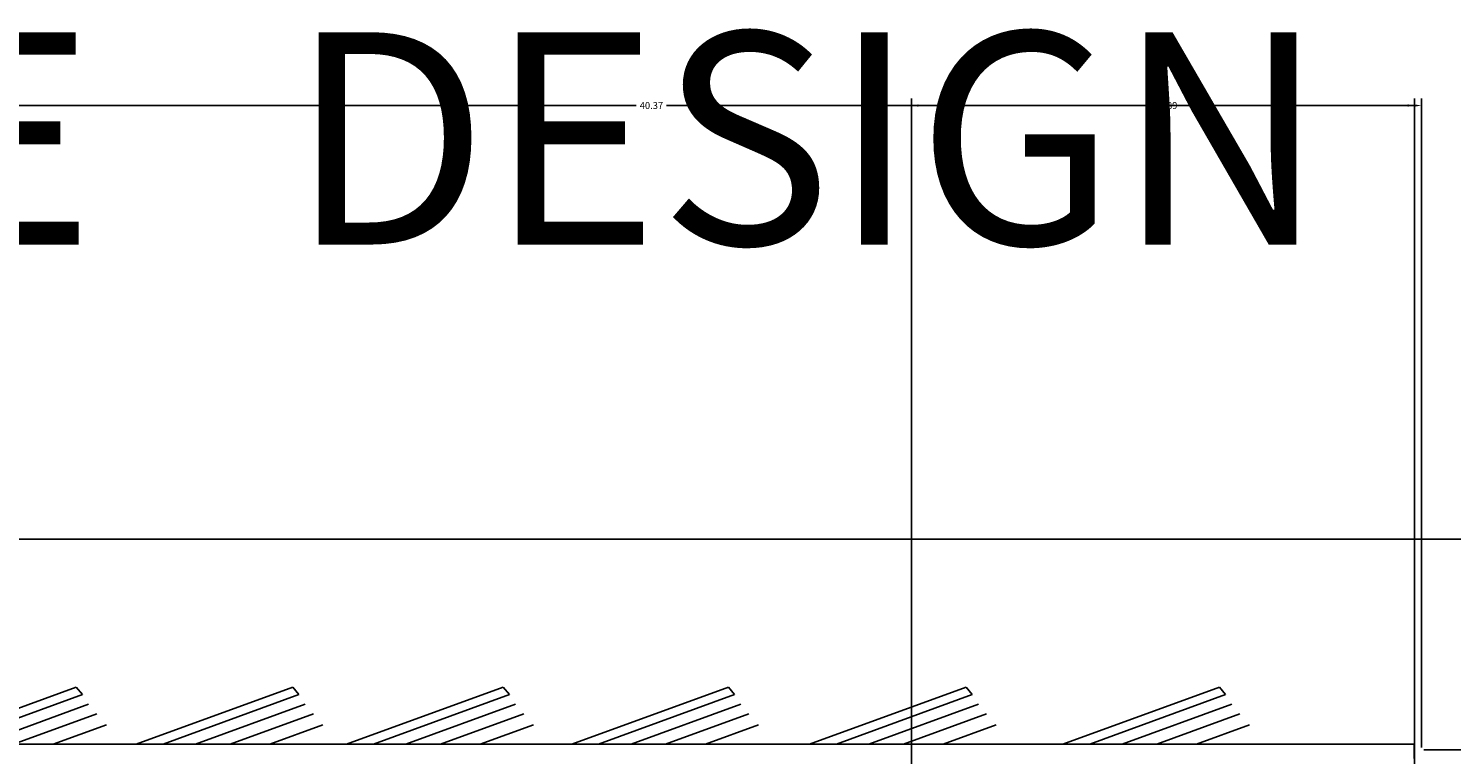
# Model space of a CAD drawing. Units: inches. Extents: x -117 to 121, y -77 to 40.
# Tile 36 of 45: x 34 to 72, y 21 to 40. Entities that reach past the tile are written whole.
import ezdxf

# ---------------------------------------------------------------- set-up
doc = ezdxf.new("R2010")
doc.units = ezdxf.units.IN
doc.header["$MEASUREMENT"] = 0
for name, color, linetype, lineweight in [('A-ANNO-DIMS', 2, 'Continuous', 18), ('A-ANNO-TEXT', 7, 'Continuous', 25), ('A-ELEV', 7, 'Continuous', 25)]:
    doc.layers.add(name, color=color, linetype=linetype, lineweight=lineweight)
doc.styles.get("Standard").update_dxf_attribs({"font": 'arial.ttf'})
doc.dimstyles.get("Standard").update_dxf_attribs({"dimtxt": 0.18, "dimasz": 0.18, "dimexe": 0.18, "dimexo": 0.0625, "dimgap": 0.09, "dimtad": 0, "dimtih": 1, "dimtoh": 1, "dimdec": 4, "dimzin": 0, "dimdsep": 46, "dimtxsty": 'Standard', "dimcen": 0.09, "dimadec": 0, "dimazin": 0, "dimtfac": 1, "dimtdec": 4, "dimtofl": 0, "dimtmove": 0, "dimatfit": 3, "dimfxl": 1, "dimtolj": 1, "dimtzin": 0, "dimarcsym": 0})

# ---------------------------------------------------------------- blocks, each defined once
blk = doc.blocks.new('*D11')
at = {"layer": 'A-ANNO-DIMS', "color": 0, "lineweight": -2, "transparency": 16777216}
for p, q in [((30.428, 21.587), (30.428, 38.61)), ((30.608, 38.43), (50.217, 38.43)), ((70.62, 38.43), (51.011, 38.43)), ((70.8, 21.604), (70.8, 38.61))]:
    blk.add_line(p, q, dxfattribs=at)
at = {"layer": 'A-ANNO-DIMS', "color": 0, "transparency": 16777216}
for points in [[(30.608, 38.46), (30.608, 38.4), (30.428, 38.43)], [(70.62, 38.46), (70.62, 38.4), (70.8, 38.43)]]:
    blk.add_solid(points, dxfattribs=at)
at = {"layer": 'Defpoints', "color": 0, "transparency": 16777216}
for p in [(70.8, 38.43), (30.428, 21.525), (70.8, 21.541)]:
    blk.add_point(p, dxfattribs=at)
at = {"layer": 'A-ANNO-DIMS', "color": 0, "transparency": 16777216, "insert": (50.614, 38.43), "char_height": 0.18, "attachment_point": 5}
blk.add_mtext('\\A1;40.37', dxfattribs=at)
blk = doc.blocks.new('*D16')
at = {"layer": 'A-ANNO-DIMS', "color": 0, "lineweight": -2, "transparency": 16777216}
for p, q in [((70.862, 21.541), (120.84, 21.541)), ((120.66, 21.361), (120.66, 9.626)), ((120.66, -2.473), (120.66, 9.262)), ((87.304, -2.653), (120.84, -2.653))]:
    blk.add_line(p, q, dxfattribs=at)
at = {"layer": 'A-ANNO-DIMS', "color": 0, "transparency": 16777216}
for points in [[(120.63, 21.361), (120.69, 21.361), (120.66, 21.541)], [(120.63, -2.473), (120.69, -2.473), (120.66, -2.653)]]:
    blk.add_solid(points, dxfattribs=at)
at = {"layer": 'Defpoints', "color": 0, "transparency": 16777216}
for p in [(70.8, 21.541), (87.242, -2.653), (120.66, -2.653)]:
    blk.add_point(p, dxfattribs=at)
at = {"layer": 'A-ANNO-DIMS', "color": 0, "transparency": 16777216, "insert": (120.66, 9.444), "char_height": 0.18, "attachment_point": 5}
blk.add_mtext('\\A1;24.194', dxfattribs=at)
blk = doc.blocks.new('*D17')
at = {"layer": 'A-ANNO-DIMS', "color": 0, "lineweight": -2, "transparency": 16777216}
for p, q in [((14.041, 27.063), (120.84, 27.063)), ((120.66, 26.883), (120.66, 24.484)), ((120.66, 21.721), (120.66, 24.12)), ((70.862, 21.541), (120.84, 21.541))]:
    blk.add_line(p, q, dxfattribs=at)
at = {"layer": 'A-ANNO-DIMS', "color": 0, "transparency": 16777216}
for points in [[(120.63, 26.883), (120.69, 26.883), (120.66, 27.063)], [(120.63, 21.721), (120.69, 21.721), (120.66, 21.541)]]:
    blk.add_solid(points, dxfattribs=at)
at = {"layer": 'Defpoints', "color": 0, "transparency": 16777216}
for p in [(13.978, 27.063), (70.8, 21.541), (120.66, 21.541)]:
    blk.add_point(p, dxfattribs=at)
at = {"layer": 'A-ANNO-DIMS', "color": 0, "transparency": 16777216, "insert": (120.66, 24.302), "char_height": 0.18, "attachment_point": 5}
blk.add_mtext('\\A1;5.522', dxfattribs=at)
blk = doc.blocks.new('*D33')
at = {"layer": 'A-ANNO-DIMS', "color": 0, "lineweight": -2, "transparency": 16777216}
for p, q in [((57.433, -43.571), (57.433, 38.61)), ((57.613, 38.43), (63.572, 38.43)), ((70.441, 38.43), (64.482, 38.43)), ((70.621, -43.571), (70.621, 38.61))]:
    blk.add_line(p, q, dxfattribs=at)
at = {"layer": 'A-ANNO-DIMS', "color": 0, "transparency": 16777216}
for points in [[(57.613, 38.46), (57.613, 38.4), (57.433, 38.43)], [(70.441, 38.46), (70.441, 38.4), (70.621, 38.43)]]:
    blk.add_solid(points, dxfattribs=at)
at = {"layer": 'Defpoints', "color": 0, "transparency": 16777216}
for p in [(70.621, 38.43), (57.433, -43.633), (70.621, -43.633)]:
    blk.add_point(p, dxfattribs=at)
at = {"layer": 'A-ANNO-DIMS', "color": 0, "transparency": 16777216, "insert": (64.027, 38.43), "char_height": 0.18, "attachment_point": 5}
blk.add_mtext('\\A1;13.189', dxfattribs=at)

msp = doc.modelspace()

# ---------------------------------------------------------------- linework, layer by layer
at = {"layer": 'A-ELEV'}
for p, q in [((31.4323, 21.689), (35.5367, 23.1855)), ((35.5367, 23.1855), (35.6986, 22.9879)), ((37.1081, 21.689), (41.2125, 23.1855)), ((41.2125, 23.1855), (41.3743, 22.9879)), ((42.6239, 21.689), (46.7283, 23.1855)), ((46.7283, 23.1855), (46.8902, 22.9879)), ((48.5258, 21.689), (52.6302, 23.1855)), ((52.6302, 23.1855), (52.7921, 22.9879)), ((54.7577, 21.689), (58.8621, 23.1855)), ((58.8621, 23.1855), (59.024, 22.9879)), ((61.3985, 21.689), (65.5029, 23.1855)), ((65.5029, 23.1855), (65.6648, 22.9879)), ((32.1361, 21.689), (35.6986, 22.9879)), ((37.8119, 21.689), (41.3743, 22.9879)), ((43.3278, 21.689), (46.8902, 22.9879)), ((49.2296, 21.689), (52.7921, 22.9879)), ((55.4616, 21.689), (59.024, 22.9879)), ((62.1024, 21.689), (65.6648, 22.9879)), ((32.9878, 21.689), (35.8604, 22.7364)), ((33.8934, 21.689), (36.0763, 22.4849)), ((38.6635, 21.689), (41.5362, 22.7364)), ((39.5692, 21.689), (41.752, 22.4849)), ((44.1794, 21.689), (47.0521, 22.7364)), ((45.085, 21.689), (47.2679, 22.4849)), ((50.0813, 21.689), (52.9539, 22.7364)), ((50.9869, 21.689), (53.1698, 22.4849)), ((56.3132, 21.689), (59.1859, 22.7364)), ((57.2188, 21.689), (59.4017, 22.4849)), ((62.954, 21.689), (65.8267, 22.7364)), ((63.8596, 21.689), (66.0425, 22.4849)), ((34.9335, 21.689), (36.3281, 22.1975)), ((40.6093, 21.689), (42.0038, 22.1975)), ((46.1251, 21.689), (47.5197, 22.1975)), ((52.027, 21.689), (53.4216, 22.1975)), ((58.2589, 21.689), (59.6535, 22.1975)), ((64.8997, 21.689), (66.2943, 22.1975)), ((30.7662, 21.689), (70.6115, 21.689)), ((70.6115, 21.689), (70.6115, 21.3104))]:
    msp.add_line(p, q, dxfattribs=at)

# ---------------------------------------------------------------- texts
at = {"layer": 'A-ANNO-TEXT'}
msp.add_text('CONCEPTUAL    GOOD   VIBE   CAFE   DESIGN', height=5.56486, dxfattribs=at).set_placement((-85.726, 34.7863))

# ---------------------------------------------------------------- dimensions: what is measured, and where the dimension line sits
at = {"layer": 'A-ANNO-DIMS'}
for base, p1, p2, override, picture, middle in [((70.8, 38.4297), (30.4277, 21.5247), (70.8, 21.5414), {"dimdec": 2, "dimlfac": 1, "dimrnd": 0, "dimzin": 0, "dimdsep": 46, "dimlunit": 2}, '*D11', (50.6138, 38.4297)), ((70.6214, 38.4297), (57.4328, -43.6334), (70.6214, -43.6334), {"dimdec": 3, "dimlfac": 1, "dimrnd": 0, "dimzin": 0, "dimdsep": 46, "dimlunit": 2}, '*D33', (64.0271, 38.4297))]:
    dim = msp.add_linear_dim(base=base, p1=p1, p2=p2, dimstyle='Standard', override=override, dxfattribs=at)
    dim.commit()
    dim.dimension.update_dxf_attribs({"geometry": picture, "text_midpoint": middle})
for base, p1, p2, picture, middle in [((120.6602, 21.5414), (13.9784, 27.0634), (70.8, 21.5414), '*D17', (120.6602, 24.3024)), ((120.6602, -2.6528), (70.8, 21.5414), (87.2416, -2.6528), '*D16', (120.6602, 9.4443))]:
    dim = msp.add_linear_dim(base=base, p1=p1, p2=p2, angle=90, dimstyle='Standard', override={"dimdec": 3, "dimlfac": 1, "dimrnd": 0, "dimzin": 0, "dimdsep": 46, "dimlunit": 2}, dxfattribs=at)
    dim.commit()
    dim.dimension.update_dxf_attribs({"geometry": picture, "text_midpoint": middle})

doc.saveas('drawing.dxf')
